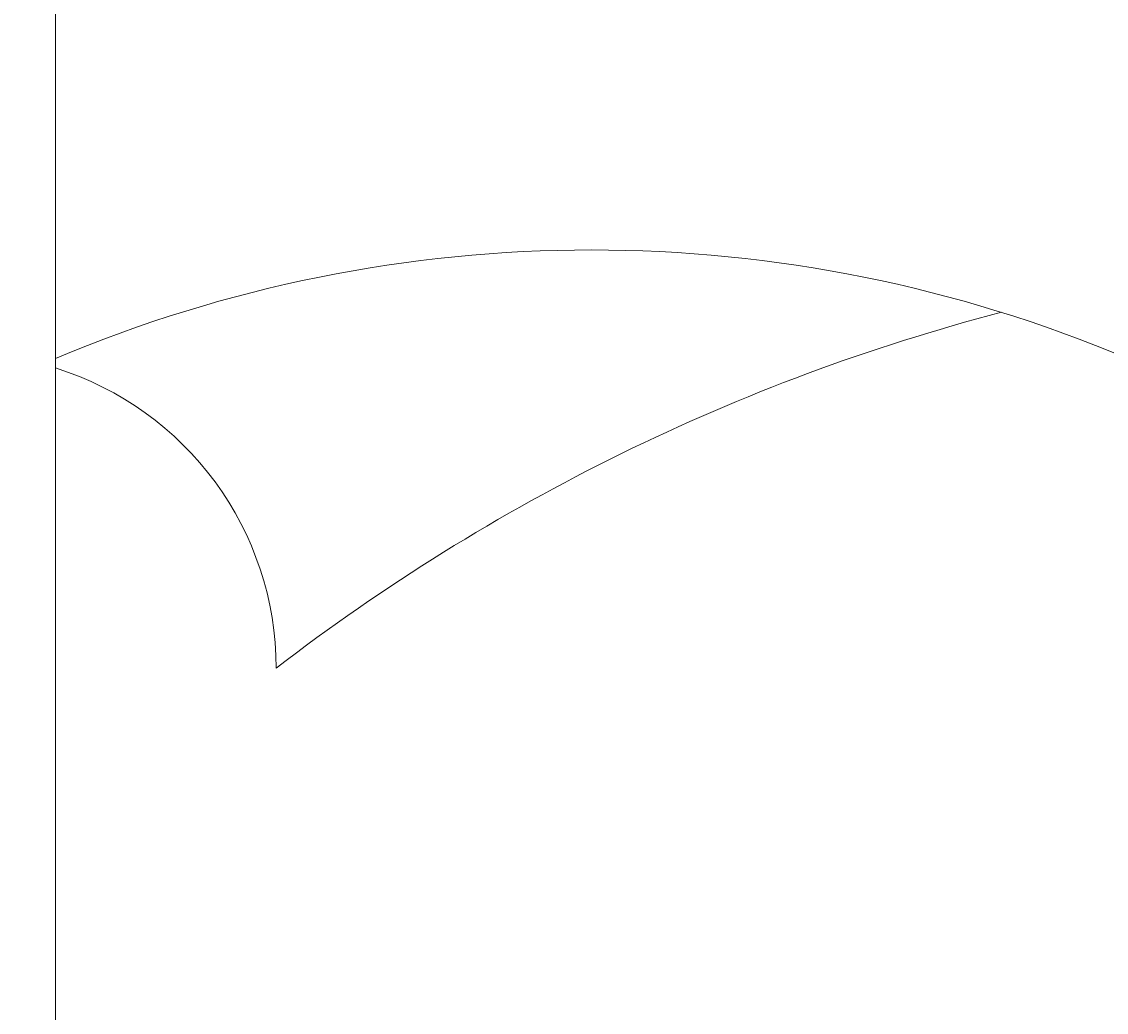
# Model space of a CAD drawing. Units: inches. Extents: x -46 to 1145, y -527 to 760.
# Tile 38 of 57: x 53 to 83, y 597 to 625. Entities that reach past the tile are written whole.
import ezdxf

# ---------------------------------------------------------------- set-up
doc = ezdxf.new("R2010")
doc.units = ezdxf.units.IN
doc.header["$MEASUREMENT"] = 0
doc.layers.add('A-ANNO-DIMS', color=2, linetype='Continuous', lineweight=18)
doc.layers.add('A-FURN', color=2, linetype='Continuous', lineweight=13)
doc.styles.get("Standard").update_dxf_attribs({"font": 'arial.ttf'})
doc.dimstyles.get("Standard").update_dxf_attribs({"dimtxt": 0.18, "dimasz": 0.18, "dimexe": 0.18, "dimexo": 0.0625, "dimgap": 0.09, "dimtad": 0, "dimtih": 1, "dimtoh": 1, "dimdec": 0, "dimzin": 0, "dimdsep": 46, "dimlunit": 3, "dimtxsty": 'Standard', "dimcen": 0.09, "dimadec": 0, "dimazin": 0, "dimtfac": 1, "dimtdec": 0, "dimtofl": 0, "dimtmove": 0, "dimatfit": 3, "dimfxl": 1, "dimtolj": 1, "dimtzin": 0, "dimarcsym": 0})

# ---------------------------------------------------------------- blocks, each defined once
blk = doc.blocks.new('BED-QUEEN-FURNISHED')
blk.add_line((0, 0), (0, 80))
for centre, radius, start, end in [((15, 13.075), 38.562, 67.1089, 112.8911), ((40.884, -5.132), 56.884, 104.6834, 127.6009), ((-2.624, 39.936), 8.8, 0, 72.6522)]:
    blk.add_arc(centre, radius, start, end)
blk = doc.blocks.new('*D685')
at = {"layer": 'A-ANNO-DIMS', "color": 0, "lineweight": -2, "transparency": 16777216}
for p, q in [((183.501, 700.889), (-46.216, 700.889)), ((-46.036, 700.709), (-46.036, 116.385)), ((-46.036, -468.302), (-46.036, 116.021)), ((12.501, -468.482), (-46.216, -468.482))]:
    blk.add_line(p, q, dxfattribs=at)
at = {"layer": 'A-ANNO-DIMS', "color": 0, "transparency": 16777216}
for points in [[(-46.066, 700.709), (-46.006, 700.709), (-46.036, 700.889)], [(-46.066, -468.302), (-46.006, -468.302), (-46.036, -468.482)]]:
    blk.add_solid(points, dxfattribs=at)
at = {"layer": 'Defpoints', "color": 0, "transparency": 16777216}
for p in [(-46.036, 700.889), (183.564, 700.889), (12.564, -468.482)]:
    blk.add_point(p, dxfattribs=at)
at = {"layer": 'A-ANNO-DIMS', "color": 0, "transparency": 16777216, "insert": (-46.036, 116.203), "char_height": 0.18, "attachment_point": 5}
blk.add_mtext('\\A1;1169.4', dxfattribs=at)

msp = doc.modelspace()

# ---------------------------------------------------------------- block references
at = {"layer": 'A-FURN'}
msp.add_blockref('BED-QUEEN-FURNISHED', (53.91, 566.503), dxfattribs=at)

# ---------------------------------------------------------------- dimensions: what is measured, and where the dimension line sits
at = {"layer": 'A-ANNO-DIMS'}
dim = msp.add_linear_dim(base=(-46.0363, 700.8886), p1=(12.5637, -468.4824), p2=(183.5637, 700.8886), angle=90, dimstyle='Standard', override={"dimdec": 1, "dimlfac": 1, "dimrnd": 0, "dimzin": 0, "dimdsep": 46, "dimlunit": 2}, dxfattribs=at)
dim.commit()
dim.dimension.update_dxf_attribs({"geometry": '*D685', "text_midpoint": (-46.0363, 116.2031)})

doc.saveas('drawing.dxf')
